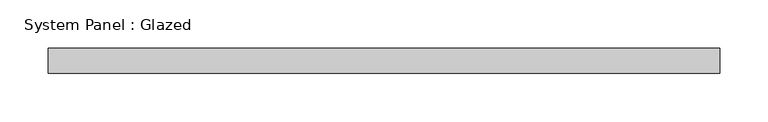
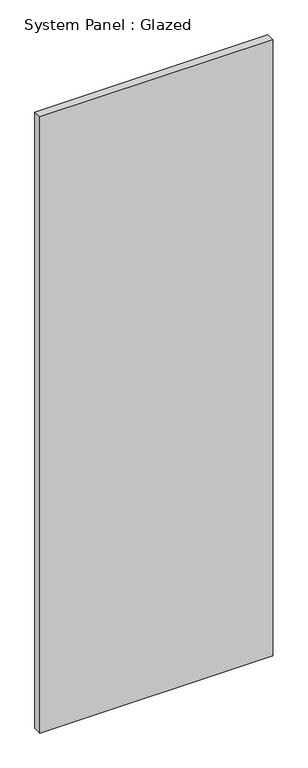
"""IFC4 building model written with IfcOpenShell, lengths in millimetres: plate geometry, System Panel : Glazed."""

from ifc_helpers import new_model, si_unit, origin, origin_with_axes, place, context, project, spatial, polyline, outline, extrude, source, transform, mapped, element, save


def system_panel_glazed_4740d582(model_context):
    return source(origin(), model_context, "Body", "SweptSolid", [
        extrude(outline(polyline([(346.075, 19.05), (-346.075, 19.05), (-346.075, 44.45), (346.075, 44.45), (346.075, 19.05)])), origin_with_axes(), (0.0, 0.0, 1.0), 1936.6147749),
    ])


if __name__ == "__main__":
    model = new_model("IFC4")
    model_context = context("Model", 3, world=origin())
    ifc_project = project(units=[si_unit("LENGTHUNIT", "METRE", prefix="MILLI")], contexts=[model_context])
    site = spatial("IfcSite", under=ifc_project)
    building = spatial("IfcBuilding", under=site)
    placement = place(None, origin())
    system_panel_glazed_shape = system_panel_glazed_4740d582(model_context)
    element("IfcPlate", 1, ObjectType="System Panel : Glazed", at=placement, inside=building, context=model_context, shape_type="MappedRepresentation", body=[
        mapped(system_panel_glazed_shape, transform((0.0, 0.0, 0.0), x_axis=(1.0, 0.0, 0.0), y_axis=(0.0, 1.0, 0.0), z_axis=(0.0, 0.0, 1.0))),
    ])
    save(model, "model.ifc")

# Revit data of these elements
# Type "System Panel : Glazed"
#   Construction Type Id = "GSP4R"
#   Analytic Construction = "1/8 in Pilkington single glazing"
#   Visual Light Transmittance = 0.9
#   Solar Heat Gain Coefficient = 0.86
#   Heat Transfer Coefficient (U) = 1.18115 BTU/(h·ft²·°F)
#   Define Thermal Properties by = 1
# Element 1 (IfcPlate, "System Panel : Glazed")
#   Materials on its faces: "Glass"
# Materials
#   "Glass": class "Glass", colour RGB 0 128 192, transparency 0.75, Description = "Soda Lime Glass", Cost = 0
